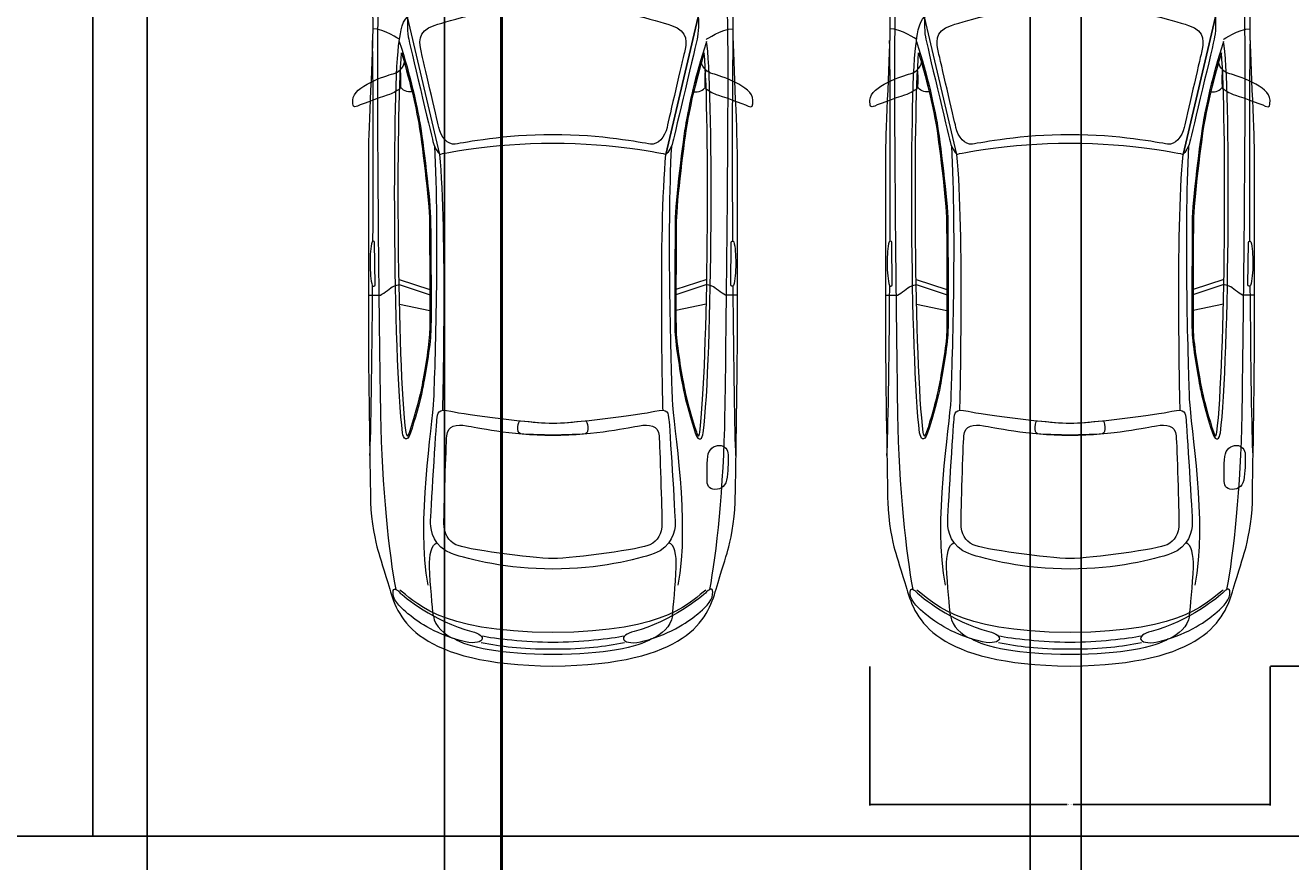
# Model space of a CAD drawing. Units: inches. Extents: x 1770 to 2988, y 1161 to 3221.
# Tile 3 of 44: x 2439 to 2663, y 1319 to 1467. Entities that reach past the tile are written whole.
import ezdxf

# ---------------------------------------------------------------- set-up
doc = ezdxf.new("R2010")
doc.units = ezdxf.units.IN
for name, color, linetype, lineweight in [('A-ANNO-DIMS', 2, 'Continuous', 18), ('AUDI', 8, 'Continuous', 13), ('C-PROP', 7, 'Continuous', 25), ('C-SITE-PAVE', 8, 'Continuous', 18)]:
    doc.layers.add(name, color=color, linetype=linetype, lineweight=lineweight)
doc.styles.get("Standard").update_dxf_attribs({"font": 'arial.ttf'})
doc.dimstyles.get("Standard").update_dxf_attribs({"dimtxt": 0.18, "dimasz": 0.18, "dimexe": 0.18, "dimexo": 0.0625, "dimgap": 0.09, "dimtad": 0, "dimtih": 1, "dimtoh": 1, "dimdec": 4, "dimzin": 0, "dimdsep": 46, "dimtxsty": 'Standard', "dimcen": 0.09, "dimadec": 0, "dimazin": 0, "dimtfac": 1, "dimtdec": 4, "dimtofl": 0, "dimtmove": 0, "dimatfit": 3, "dimfxl": 1, "dimtolj": 1, "dimtzin": 0, "dimarcsym": 0})

# ---------------------------------------------------------------- blocks, each defined once
blk = doc.blocks.new('CAR-SEDAN-PLAN')
for points, knots in [([(35.35, 0), (11.45, 0.26), (7.98, 8.3), (6.52, 13.59), (6.52, 13.59), (5.56, 16.72), (4.79, 19.21), (4.41, 20.48), (4.41, 20.48), (4.03, 21.76), (3.2, 25.65), (3.14, 28.9), (3.14, 28.9), (3.07, 32.16), (2.76, 51.56), (2.76, 56.91), (2.76, 56.91), (2.76, 62.27), (2.76, 87.35), (2.76, 90.92), (2.76, 90.92), (2.76, 94.49), (3.52, 108.72), (3.52, 113.25), (3.52, 113.25), (3.52, 117.78), (2.76, 123.46), (2.76, 125.81), (2.76, 125.81), (2.76, 128.17), (3.2, 140.62), (3.39, 143.36), (3.39, 143.36), (3.58, 146.1), (4.61, 147.66), (5.5, 149.61), (5.5, 149.61), (8.94, 157.2), (17.74, 161.35), (18.69, 161.99), (18.69, 161.99), (19.65, 162.63), (20.67, 162.97), (21.88, 162.97), (21.88, 162.97), (23.1, 162.97), (23.41, 162.37), (23.92, 162.5), (23.92, 162.5), (24.43, 162.63), (25.7, 162.97), (27.11, 162.97), (27.11, 162.97), (28.52, 162.97), (35.35, 162.97), (35.35, 162.97), (35.35, 162.97), (35.35, 162.97), (42.18, 162.97), (43.59, 162.97), (43.59, 162.97), (45, 162.97), (46.27, 162.63), (46.78, 162.5), (46.78, 162.5), (47.29, 162.37), (47.6, 162.97), (48.82, 162.97), (48.82, 162.97), (50.04, 162.97), (51.05, 162.63), (52.01, 161.99), (52.01, 161.99), (52.96, 161.35), (61.76, 157.2), (65.21, 149.61), (65.21, 149.61), (66.09, 147.66), (67.12, 146.1), (67.31, 143.36), (67.31, 143.36), (67.5, 140.62), (67.95, 128.17), (67.95, 125.81), (67.95, 125.81), (67.95, 123.46), (67.18, 117.78), (67.18, 113.25), (67.18, 113.25), (67.18, 108.72), (67.95, 94.49), (67.95, 90.92), (67.95, 90.92), (67.95, 87.35), (67.95, 62.27), (67.95, 56.91), (67.95, 56.91), (67.95, 51.56), (67.63, 32.16), (67.57, 28.9), (67.57, 28.9), (67.5, 25.65), (66.67, 21.76), (66.29, 20.48), (66.29, 20.48), (65.91, 19.21), (65.14, 16.72), (64.19, 13.59), (64.19, 13.59), (62.72, 8.3), (59.25, 0.26), (35.35, 0)], [0, 0, 0, 0, 0.035714, 0.035714, 0.035714, 0.035714, 0.071429, 0.071429, 0.071429, 0.071429, 0.107143, 0.107143, 0.107143, 0.107143, 0.142857, 0.142857, 0.142857, 0.142857, 0.178571, 0.178571, 0.178571, 0.178571, 0.214286, 0.214286, 0.214286, 0.214286, 0.25, 0.25, 0.25, 0.25, 0.285714, 0.285714, 0.285714, 0.285714, 0.321429, 0.321429, 0.321429, 0.321429, 0.357143, 0.357143, 0.357143, 0.357143, 0.392857, 0.392857, 0.392857, 0.392857, 0.428571, 0.428571, 0.428571, 0.428571, 0.464286, 0.464286, 0.464286, 0.464286, 0.5, 0.5, 0.5, 0.5, 0.535714, 0.535714, 0.535714, 0.535714, 0.571429, 0.571429, 0.571429, 0.571429, 0.607143, 0.607143, 0.607143, 0.607143, 0.642857, 0.642857, 0.642857, 0.642857, 0.678571, 0.678571, 0.678571, 0.678571, 0.714286, 0.714286, 0.714286, 0.714286, 0.75, 0.75, 0.75, 0.75, 0.785714, 0.785714, 0.785714, 0.785714, 0.821429, 0.821429, 0.821429, 0.821429, 0.857143, 0.857143, 0.857143, 0.857143, 0.892857, 0.892857, 0.892857, 0.892857, 0.928571, 0.928571, 0.928571, 0.928571, 0.964286, 0.964286, 0.964286, 0.964286, 1, 1, 1, 1]), ([(7.64, 13.52), (6.44, 19.53), (5.16, 31.7), (4.94, 44.37), (4.94, 44.37), (4.72, 57.04), (4.17, 105.75), (4.5, 116.02), (4.5, 116.02), (4.83, 126.28), (5.01, 139.24), (6.83, 148.05)], [0, 0, 0, 0, 0.333333, 0.333333, 0.333333, 0.333333, 0.666667, 0.666667, 0.666667, 0.666667, 1, 1, 1, 1]), ([(63.07, 13.52), (64.27, 19.53), (65.54, 31.7), (65.76, 44.37), (65.76, 44.37), (65.98, 57.04), (66.53, 105.75), (66.2, 116.02), (66.2, 116.02), (65.87, 126.28), (65.69, 139.24), (63.87, 148.05)], [0, 0, 0, 0, 0.333333, 0.333333, 0.333333, 0.333333, 0.666667, 0.666667, 0.666667, 0.666667, 1, 1, 1, 1]), ([(35.35, 92.33), (46.17, 92.33), (55.33, 90.37), (55.33, 90.37), (55.33, 90.37), (55.33, 90.37), (61.04, 114.67), (61.04, 114.67), (61.04, 114.67), (58.76, 116.14), (55.78, 121.11), (35.35, 121.11), (35.35, 121.11), (14.92, 121.11), (11.94, 116.14), (9.66, 114.67), (9.66, 114.67), (9.66, 114.67), (15.37, 90.37), (15.37, 90.37), (15.37, 90.37), (15.37, 90.37), (24.53, 92.33), (35.35, 92.33)], [0, 0, 0, 0, 0.166667, 0.166667, 0.166667, 0.166667, 0.333333, 0.333333, 0.333333, 0.333333, 0.5, 0.5, 0.5, 0.5, 0.666667, 0.666667, 0.666667, 0.666667, 0.833333, 0.833333, 0.833333, 0.833333, 1, 1, 1, 1]), ([(35.35, 92.33), (46.17, 92.33), (55.33, 90.37), (55.33, 90.37), (55.33, 90.37), (55.33, 90.37), (61.04, 114.67), (61.04, 114.67), (61.04, 114.67), (58.76, 116.14), (55.78, 121.11), (35.35, 121.11), (35.35, 121.11), (14.92, 121.11), (11.94, 116.14), (9.66, 114.67), (9.66, 114.67), (9.66, 114.67), (15.37, 90.37), (15.37, 90.37), (15.37, 90.37), (15.37, 90.37), (24.53, 92.33), (35.35, 92.33)], [0, 0, 0, 0, 0.166667, 0.166667, 0.166667, 0.166667, 0.333333, 0.333333, 0.333333, 0.333333, 0.5, 0.5, 0.5, 0.5, 0.666667, 0.666667, 0.666667, 0.666667, 0.833333, 0.833333, 0.833333, 0.833333, 1, 1, 1, 1]), ([(9.66, 114.67), (9.66, 114.67), (15.37, 90.37), (15.37, 90.37), (15.37, 90.37), (15.37, 90.37), (14.48, 91.26), (14.15, 92.64), (14.15, 92.64), (13.82, 94.03), (10.04, 109.86), (9.79, 111.17), (9.79, 111.17), (9.55, 112.47), (9.66, 114.67), (9.66, 114.67)], [0, 0, 0, 0, 0.25, 0.25, 0.25, 0.25, 0.5, 0.5, 0.5, 0.5, 0.75, 0.75, 0.75, 0.75, 1, 1, 1, 1]), ([(9.66, 114.67), (9.66, 114.67), (15.37, 90.37), (15.37, 90.37), (15.37, 90.37), (15.37, 90.37), (14.48, 91.26), (14.15, 92.64), (14.15, 92.64), (13.82, 94.03), (10.04, 109.86), (9.79, 111.17), (9.79, 111.17), (9.55, 112.47), (9.66, 114.67), (9.66, 114.67)], [0, 0, 0, 0, 0.25, 0.25, 0.25, 0.25, 0.5, 0.5, 0.5, 0.5, 0.75, 0.75, 0.75, 0.75, 1, 1, 1, 1]), ([(35.35, 93.86), (43.94, 93.86), (50.97, 92.45), (52.59, 92.2), (52.59, 92.2), (53.92, 92), (55.15, 93.44), (55.52, 95.16), (55.52, 95.16), (55.89, 96.88), (58.26, 106.94), (58.59, 108.38), (58.59, 108.38), (58.92, 109.82), (59.47, 112.19), (56.31, 113.17), (56.31, 113.17), (53.15, 114.15), (47.56, 116.15), (35.35, 116.15), (35.35, 116.15), (23.15, 116.15), (17.55, 114.15), (14.39, 113.17), (14.39, 113.17), (11.23, 112.19), (11.79, 109.82), (12.11, 108.38), (12.11, 108.38), (12.44, 106.94), (14.81, 96.88), (15.18, 95.16), (15.18, 95.16), (15.55, 93.44), (16.78, 92), (18.11, 92.2), (18.11, 92.2), (19.74, 92.45), (26.76, 93.86), (35.35, 93.86)], [0, 0, 0, 0, 0.1, 0.1, 0.1, 0.1, 0.2, 0.2, 0.2, 0.2, 0.3, 0.3, 0.3, 0.3, 0.4, 0.4, 0.4, 0.4, 0.5, 0.5, 0.5, 0.5, 0.6, 0.6, 0.6, 0.6, 0.7, 0.7, 0.7, 0.7, 0.8, 0.8, 0.8, 0.8, 0.9, 0.9, 0.9, 0.9, 1, 1, 1, 1]), ([(61.04, 114.67), (61.04, 114.67), (55.33, 90.37), (55.33, 90.37), (55.33, 90.37), (55.33, 90.37), (56.23, 91.26), (56.55, 92.64), (56.55, 92.64), (56.88, 94.03), (60.66, 109.86), (60.91, 111.17), (60.91, 111.17), (61.15, 112.47), (61.04, 114.67), (61.04, 114.67)], [0, 0, 0, 0, 0.25, 0.25, 0.25, 0.25, 0.5, 0.5, 0.5, 0.5, 0.75, 0.75, 0.75, 0.75, 1, 1, 1, 1]), ([(8.78, 41.21), (8.91, 40.21), (9.53, 39.31), (10.19, 41.21), (10.19, 41.21), (10.85, 43.12), (11.93, 47.01), (12.26, 48.66), (12.26, 48.66), (12.59, 50.32), (13.58, 55.79), (13.75, 58.52), (13.75, 58.52), (13.92, 61.25), (13.75, 75.25), (13.75, 78.56), (13.75, 78.56), (13.75, 81.87), (12.34, 93.22), (11.85, 95.95), (11.85, 95.95), (11.35, 98.68), (10.27, 104.15), (8.2, 110.31), (8.2, 110.31), (6.96, 103.49), (7.13, 54.21), (8.78, 41.21)], [0, 0, 0, 0, 0.142857, 0.142857, 0.142857, 0.142857, 0.285714, 0.285714, 0.285714, 0.285714, 0.428571, 0.428571, 0.428571, 0.428571, 0.571429, 0.571429, 0.571429, 0.571429, 0.714286, 0.714286, 0.714286, 0.714286, 0.857143, 0.857143, 0.857143, 0.857143, 1, 1, 1, 1]), ([(61.92, 41.21), (61.79, 40.21), (61.17, 39.31), (60.51, 41.21), (60.51, 41.21), (59.85, 43.12), (58.77, 47.01), (58.44, 48.66), (58.44, 48.66), (58.11, 50.32), (57.12, 55.79), (56.95, 58.52), (56.95, 58.52), (56.79, 61.25), (56.95, 75.25), (56.95, 78.56), (56.95, 78.56), (56.95, 81.87), (58.36, 93.22), (58.86, 95.95), (58.86, 95.95), (59.35, 98.68), (60.43, 104.15), (62.5, 110.31), (62.5, 110.31), (63.74, 103.49), (63.57, 54.21), (61.92, 41.21)], [0, 0, 0, 0, 0.142857, 0.142857, 0.142857, 0.142857, 0.285714, 0.285714, 0.285714, 0.285714, 0.428571, 0.428571, 0.428571, 0.428571, 0.571429, 0.571429, 0.571429, 0.571429, 0.714286, 0.714286, 0.714286, 0.714286, 0.857143, 0.857143, 0.857143, 0.857143, 1, 1, 1, 1]), ([(9.41, 41.26), (9.41, 41.26), (9.41, 41.26), (9.41, 41.26), (9.41, 41.26), (9.46, 40.9), (9.56, 40.69), (9.63, 40.58), (9.63, 40.58), (9.71, 40.67), (9.84, 40.87), (10, 41.35), (10, 41.35), (10.65, 43.21), (11.72, 47.08), (12.06, 48.75), (12.06, 48.75), (12.46, 50.75), (13.39, 55.99), (13.54, 58.54), (13.54, 58.54), (13.66, 60.54), (13.6, 68.71), (13.56, 74.11), (13.56, 74.11), (13.56, 74.11), (13.54, 78.56), (13.54, 78.56), (13.54, 78.56), (13.54, 81.86), (12.12, 93.26), (11.64, 95.88), (11.64, 95.88), (10.85, 100.24), (9.82, 104.4), (8.6, 108.3), (8.6, 108.3), (7.63, 97), (7.88, 53.31), (9.41, 41.26)], [0, 0, 0, 0, 0.1, 0.1, 0.1, 0.1, 0.2, 0.2, 0.2, 0.2, 0.3, 0.3, 0.3, 0.3, 0.4, 0.4, 0.4, 0.4, 0.5, 0.5, 0.5, 0.5, 0.6, 0.6, 0.6, 0.6, 0.7, 0.7, 0.7, 0.7, 0.8, 0.8, 0.8, 0.8, 0.9, 0.9, 0.9, 0.9, 1, 1, 1, 1]), ([(61.29, 41.26), (61.29, 41.26), (61.29, 41.26), (61.29, 41.26), (61.29, 41.26), (61.24, 40.9), (61.14, 40.69), (61.07, 40.58), (61.07, 40.58), (60.99, 40.67), (60.86, 40.87), (60.7, 41.35), (60.7, 41.35), (60.05, 43.21), (58.98, 47.08), (58.64, 48.75), (58.64, 48.75), (58.24, 50.75), (57.32, 55.99), (57.16, 58.54), (57.16, 58.54), (57.04, 60.54), (57.1, 68.71), (57.14, 74.11), (57.14, 74.11), (57.14, 74.11), (57.16, 78.56), (57.16, 78.56), (57.16, 78.56), (57.16, 81.86), (58.59, 93.26), (59.06, 95.88), (59.06, 95.88), (59.85, 100.24), (60.88, 104.4), (62.1, 108.3), (62.1, 108.3), (63.07, 97), (62.82, 53.31), (61.29, 41.26)], [0, 0, 0, 0, 0.1, 0.1, 0.1, 0.1, 0.2, 0.2, 0.2, 0.2, 0.3, 0.3, 0.3, 0.3, 0.4, 0.4, 0.4, 0.4, 0.5, 0.5, 0.5, 0.5, 0.6, 0.6, 0.6, 0.6, 0.7, 0.7, 0.7, 0.7, 0.8, 0.8, 0.8, 0.8, 0.9, 0.9, 0.9, 0.9, 1, 1, 1, 1]), ([(8.34, 105.29), (8.03, 105), (7.63, 104.75), (7.11, 104.61), (7.11, 104.61), (5.83, 104.26), (0.07, 102.46), (0, 99.98), (0, 99.98), (0, 98.93), (0.02, 98.57), (0.85, 98.93), (0.85, 98.93), (1.67, 99.3), (5.81, 100.79), (6.5, 100.99), (6.5, 100.99), (7.13, 101.18), (8.06, 101.74), (8.4, 102.11), (8.4, 102.11), (8.48, 103.13), (8.47, 104.61), (8.34, 105.29)], [0, 0, 0, 0, 0.166667, 0.166667, 0.166667, 0.166667, 0.333333, 0.333333, 0.333333, 0.333333, 0.5, 0.5, 0.5, 0.5, 0.666667, 0.666667, 0.666667, 0.666667, 0.833333, 0.833333, 0.833333, 0.833333, 1, 1, 1, 1]), ([(8.34, 105.29), (8.47, 104.61), (8.48, 103.13), (8.4, 102.11), (8.4, 102.11), (8.43, 102.14), (8.47, 102.18), (8.49, 102.2), (8.49, 102.2), (8.67, 101.82), (9.61, 101.3), (10.48, 101.44), (10.48, 101.44), (10.36, 101.92), (9.1, 106.66), (9.1, 106.66), (9.1, 106.66), (9.05, 106.27), (8.8, 105.73), (8.34, 105.29)], [0, 0, 0, 0, 0.2, 0.2, 0.2, 0.2, 0.4, 0.4, 0.4, 0.4, 0.6, 0.6, 0.6, 0.6, 0.8, 0.8, 0.8, 0.8, 1, 1, 1, 1]), ([(62.36, 105.29), (62.23, 104.61), (62.22, 103.13), (62.3, 102.11), (62.3, 102.11), (62.27, 102.14), (62.24, 102.18), (62.22, 102.2), (62.22, 102.2), (62.03, 101.82), (61.09, 101.3), (60.22, 101.44), (60.22, 101.44), (60.34, 101.92), (61.6, 106.66), (61.6, 106.66), (61.6, 106.66), (61.66, 106.27), (61.9, 105.73), (62.36, 105.29)], [0, 0, 0, 0, 0.2, 0.2, 0.2, 0.2, 0.4, 0.4, 0.4, 0.4, 0.6, 0.6, 0.6, 0.6, 0.8, 0.8, 0.8, 0.8, 1, 1, 1, 1]), ([(62.36, 105.29), (62.67, 105), (63.07, 104.75), (63.59, 104.61), (63.59, 104.61), (64.87, 104.26), (70.63, 102.46), (70.7, 99.98), (70.7, 99.98), (70.7, 98.93), (70.68, 98.57), (69.86, 98.93), (69.86, 98.93), (69.03, 99.3), (64.89, 100.79), (64.21, 100.99), (64.21, 100.99), (63.57, 101.18), (62.64, 101.74), (62.3, 102.11), (62.3, 102.11), (62.22, 103.13), (62.23, 104.61), (62.36, 105.29)], [0, 0, 0, 0, 0.166667, 0.166667, 0.166667, 0.166667, 0.333333, 0.333333, 0.333333, 0.333333, 0.5, 0.5, 0.5, 0.5, 0.666667, 0.666667, 0.666667, 0.666667, 0.833333, 0.833333, 0.833333, 0.833333, 1, 1, 1, 1]), ([(14.41, 91.86), (15.27, 76.4), (14.46, 52.09), (14.27, 47.16), (14.27, 47.16), (14.09, 42.23), (11.07, 25.47), (13.28, 14.26)], [0, 0, 0, 0, 0.5, 0.5, 0.5, 0.5, 1, 1, 1, 1]), ([(56.29, 91.86), (55.44, 76.4), (56.24, 52.09), (56.43, 47.16), (56.43, 47.16), (56.61, 42.23), (59.63, 25.47), (57.42, 14.26)], [0, 0, 0, 0, 0.5, 0.5, 0.5, 0.5, 1, 1, 1, 1]), ([(3.92, 67.36), (3.92, 67.07), (3.53, 66.96), (3.44, 67.25), (3.44, 67.25), (3.17, 68.09), (3.04, 69.59), (3.04, 71.09), (3.04, 71.09), (3.04, 72.59), (3.13, 74.05), (3.39, 74.92), (3.39, 74.92), (3.48, 75.18), (3.84, 75.11), (3.84, 74.81), (3.84, 74.81), (3.84, 74.81), (3.92, 67.36), (3.92, 67.36)], [0, 0, 0, 0, 0.2, 0.2, 0.2, 0.2, 0.4, 0.4, 0.4, 0.4, 0.6, 0.6, 0.6, 0.6, 0.8, 0.8, 0.8, 0.8, 1, 1, 1, 1]), ([(66.78, 67.36), (66.78, 67.07), (67.18, 66.96), (67.27, 67.25), (67.27, 67.25), (67.53, 68.09), (67.66, 69.59), (67.66, 71.09), (67.66, 71.09), (67.66, 72.59), (67.58, 74.05), (67.31, 74.92), (67.31, 74.92), (67.22, 75.18), (66.87, 75.11), (66.87, 74.81), (66.87, 74.81), (66.87, 74.81), (66.78, 67.36), (66.78, 67.36)], [0, 0, 0, 0, 0.2, 0.2, 0.2, 0.2, 0.4, 0.4, 0.4, 0.4, 0.6, 0.6, 0.6, 0.6, 0.8, 0.8, 0.8, 0.8, 1, 1, 1, 1]), ([(2.76, 65.49), (2.76, 65.49), (4.19, 65.49), (4.66, 65.49), (4.66, 65.49), (5.14, 65.49), (6.39, 66.63), (6.96, 66.97), (6.96, 66.97), (7.54, 67.3), (8.17, 67.38), (8.17, 67.38)], [0, 0, 0, 0, 0.333333, 0.333333, 0.333333, 0.333333, 0.666667, 0.666667, 0.666667, 0.666667, 1, 1, 1, 1]), ([(67.95, 65.49), (67.95, 65.49), (66.51, 65.49), (66.04, 65.49), (66.04, 65.49), (65.57, 65.49), (64.32, 66.63), (63.74, 66.97), (63.74, 66.97), (63.16, 67.3), (62.53, 67.38), (62.53, 67.38)], [0, 0, 0, 0, 0.333333, 0.333333, 0.333333, 0.333333, 0.666667, 0.666667, 0.666667, 0.666667, 1, 1, 1, 1]), ([(35.35, 17.14), (43.39, 17.14), (50.14, 18.76), (53.24, 19.87), (53.24, 19.87), (56.34, 20.99), (56.96, 23.85), (56.96, 25.27), (56.96, 25.27), (56.96, 26.7), (55.97, 42.4), (55.85, 43.52), (55.85, 43.52), (55.72, 44.63), (55.78, 45.63), (53.36, 45.01), (53.36, 45.01), (50.95, 44.39), (38.36, 42.9), (35.35, 42.9), (35.35, 42.9), (32.35, 42.9), (19.76, 44.39), (17.34, 45.01), (17.34, 45.01), (14.92, 45.63), (14.98, 44.63), (14.86, 43.52), (14.86, 43.52), (14.73, 42.4), (13.74, 26.7), (13.74, 25.27), (13.74, 25.27), (13.74, 23.85), (14.36, 20.99), (17.46, 19.87), (17.46, 19.87), (20.56, 18.76), (27.32, 17.14), (35.35, 17.14)], [0, 0, 0, 0, 0.1, 0.1, 0.1, 0.1, 0.2, 0.2, 0.2, 0.2, 0.3, 0.3, 0.3, 0.3, 0.4, 0.4, 0.4, 0.4, 0.5, 0.5, 0.5, 0.5, 0.6, 0.6, 0.6, 0.6, 0.7, 0.7, 0.7, 0.7, 0.8, 0.8, 0.8, 0.8, 0.9, 0.9, 0.9, 0.9, 1, 1, 1, 1]), ([(35.35, 17.14), (43.39, 17.14), (50.14, 18.76), (53.24, 19.87), (53.24, 19.87), (56.34, 20.99), (56.96, 23.85), (56.96, 25.27), (56.96, 25.27), (56.96, 26.7), (55.97, 42.4), (55.85, 43.52), (55.85, 43.52), (55.72, 44.63), (55.78, 45.63), (53.36, 45.01), (53.36, 45.01), (50.95, 44.39), (38.36, 42.9), (35.35, 42.9), (35.35, 42.9), (32.35, 42.9), (19.76, 44.39), (17.34, 45.01), (17.34, 45.01), (14.92, 45.63), (14.98, 44.63), (14.86, 43.52), (14.86, 43.52), (14.73, 42.4), (13.74, 26.7), (13.74, 25.27), (13.74, 25.27), (13.74, 23.85), (14.36, 20.99), (17.46, 19.87), (17.46, 19.87), (20.56, 18.76), (27.32, 17.14), (35.35, 17.14)], [0, 0, 0, 0, 0.1, 0.1, 0.1, 0.1, 0.2, 0.2, 0.2, 0.2, 0.3, 0.3, 0.3, 0.3, 0.4, 0.4, 0.4, 0.4, 0.5, 0.5, 0.5, 0.5, 0.6, 0.6, 0.6, 0.6, 0.7, 0.7, 0.7, 0.7, 0.8, 0.8, 0.8, 0.8, 0.9, 0.9, 0.9, 0.9, 1, 1, 1, 1]), ([(35.35, 19), (39.16, 19), (51.13, 20.68), (52.5, 21.43), (52.5, 21.43), (53.86, 22.17), (54.61, 23.22), (54.61, 25.27), (54.61, 25.27), (54.61, 27.32), (54.23, 38.8), (54.11, 40.66), (54.11, 40.66), (53.99, 42.52), (52.31, 42.71), (50.64, 42.46), (50.64, 42.46), (48.96, 42.21), (43.07, 40.79), (35.35, 40.79), (35.35, 40.79), (27.63, 40.79), (21.74, 42.21), (20.07, 42.46), (20.07, 42.46), (18.39, 42.71), (16.72, 42.52), (16.59, 40.66), (16.59, 40.66), (16.47, 38.8), (16.1, 27.32), (16.1, 25.27), (16.1, 25.27), (16.1, 23.22), (16.84, 22.17), (18.21, 21.43), (18.21, 21.43), (19.57, 20.68), (31.54, 19), (35.35, 19)], [0, 0, 0, 0, 0.1, 0.1, 0.1, 0.1, 0.2, 0.2, 0.2, 0.2, 0.3, 0.3, 0.3, 0.3, 0.4, 0.4, 0.4, 0.4, 0.5, 0.5, 0.5, 0.5, 0.6, 0.6, 0.6, 0.6, 0.7, 0.7, 0.7, 0.7, 0.8, 0.8, 0.8, 0.8, 0.9, 0.9, 0.9, 0.9, 1, 1, 1, 1]), ([(35.35, 40.79), (35.35, 40.79), (39.9, 40.87), (41.09, 41.04), (41.09, 41.04), (41.83, 41.15), (41.48, 43.37), (41.13, 43.34), (41.13, 43.34), (38.95, 43.13), (37.12, 42.9), (35.35, 42.9), (35.35, 42.9), (33.58, 42.9), (31.75, 43.13), (29.57, 43.34), (29.57, 43.34), (29.22, 43.37), (28.87, 41.15), (29.61, 41.04), (29.61, 41.04), (30.8, 40.87), (35.35, 40.79), (35.35, 40.79)], [0, 0, 0, 0, 0.166667, 0.166667, 0.166667, 0.166667, 0.333333, 0.333333, 0.333333, 0.333333, 0.5, 0.5, 0.5, 0.5, 0.666667, 0.666667, 0.666667, 0.666667, 0.833333, 0.833333, 0.833333, 0.833333, 1, 1, 1, 1]), ([(62.61, 32.88), (62.53, 32.07), (62.82, 31.23), (63.99, 31.2), (63.99, 31.2), (65.17, 31.18), (65.98, 31.81), (66.15, 33.36), (66.15, 33.36), (66.32, 34.92), (66.32, 36.47), (66.32, 37.33), (66.32, 37.33), (66.32, 38.2), (65.72, 38.97), (64.77, 38.97), (64.77, 38.97), (63.82, 38.97), (62.87, 38.37), (62.7, 36.99), (62.7, 36.99), (62.53, 35.61), (62.61, 32.88), (62.61, 32.88)], [0, 0, 0, 0, 0.166667, 0.166667, 0.166667, 0.166667, 0.333333, 0.333333, 0.333333, 0.333333, 0.5, 0.5, 0.5, 0.5, 0.666667, 0.666667, 0.666667, 0.666667, 0.833333, 0.833333, 0.833333, 0.833333, 1, 1, 1, 1]), ([(14.24, 8.87), (14.05, 10.4), (13.69, 14.31), (13.55, 17.48), (13.55, 17.48), (13.46, 19.63), (13.92, 21.53), (14.85, 21.79)], [0, 0, 0, 0, 0.5, 0.5, 0.5, 0.5, 1, 1, 1, 1]), ([(56.46, 8.87), (56.65, 10.4), (57.01, 14.31), (57.15, 17.48), (57.15, 17.48), (57.24, 19.63), (56.78, 21.53), (55.85, 21.79)], [0, 0, 0, 0, 0.5, 0.5, 0.5, 0.5, 1, 1, 1, 1]), ([(21, 6.11), (14.38, 7.82), (9.01, 12.29), (8.18, 13.09), (8.18, 13.09), (7.46, 13.8), (7.01, 13.87), (7.12, 12.63), (7.12, 12.63), (7.23, 11.4), (8.78, 10.02), (9.74, 9.23), (9.74, 9.23), (10.95, 8.22), (14.29, 5.7), (19.21, 4.45), (19.21, 4.45), (21.09, 3.91), (22.44, 4.09), (22.8, 4.63), (22.8, 4.63), (23.15, 5.17), (22.32, 5.76), (21, 6.11)], [0, 0, 0, 0, 0.166667, 0.166667, 0.166667, 0.166667, 0.333333, 0.333333, 0.333333, 0.333333, 0.5, 0.5, 0.5, 0.5, 0.666667, 0.666667, 0.666667, 0.666667, 0.833333, 0.833333, 0.833333, 0.833333, 1, 1, 1, 1]), ([(62.4, 13.43), (60.03, 11.81), (55.98, 5.94), (35.35, 5.94), (35.35, 5.94), (14.73, 5.94), (10.67, 11.81), (8.3, 13.43)], [0, 0, 0, 0, 0.5, 0.5, 0.5, 0.5, 1, 1, 1, 1]), ([(49.7, 6.11), (56.32, 7.82), (61.69, 12.29), (62.52, 13.09), (62.52, 13.09), (63.25, 13.8), (63.69, 13.87), (63.58, 12.63), (63.58, 12.63), (63.47, 11.4), (61.92, 10.02), (60.97, 9.23), (60.97, 9.23), (59.75, 8.22), (56.42, 5.7), (51.49, 4.45), (51.49, 4.45), (49.61, 3.91), (48.26, 4.09), (47.91, 4.63), (47.91, 4.63), (47.55, 5.17), (48.38, 5.76), (49.7, 6.11)], [0, 0, 0, 0, 0.166667, 0.166667, 0.166667, 0.166667, 0.333333, 0.333333, 0.333333, 0.333333, 0.5, 0.5, 0.5, 0.5, 0.666667, 0.666667, 0.666667, 0.666667, 0.833333, 0.833333, 0.833333, 0.833333, 1, 1, 1, 1]), ([(52.75, 4.81), (50.45, 3.34), (44.44, 2.03), (35.35, 2.03), (35.35, 2.03), (26.26, 2.03), (20.25, 3.34), (17.95, 4.81)], [0, 0, 0, 0, 0.5, 0.5, 0.5, 0.5, 1, 1, 1, 1]), ([(48.01, 5.28), (45.61, 4.83), (40.16, 4.17), (35.35, 4.17), (35.35, 4.17), (30.54, 4.17), (25.09, 4.83), (22.7, 5.28)], [0, 0, 0, 0, 0.5, 0.5, 0.5, 0.5, 1, 1, 1, 1]), ([(48.01, 4.08), (44.31, 3.43), (41.37, 2.96), (35.35, 2.96), (35.35, 2.96), (29.33, 2.96), (26.39, 3.43), (22.7, 4.08)], [0, 0, 0, 0, 0.5, 0.5, 0.5, 0.5, 1, 1, 1, 1])]:
    blk.add_open_spline(points, degree=3, knots=knots)
for points in [[(8.16, 109.91), (8.28, 111.03), (8.55, 113.81), (9.66, 114.67)], [(8.25, 110.69), (8.25, 110.69), (5.57, 112.58), (3.51, 112.58)], [(62.45, 110.69), (62.45, 110.69), (65.13, 112.58), (67.19, 112.58)], [(3.55, 75.07), (3.63, 89.88), (3.62, 104.6), (3.47, 110.53)], [(67.15, 75.07), (67.07, 89.88), (67.08, 104.6), (67.23, 110.53)], [(15.89, 45.19), (15.89, 45.19), (16.68, 76.85), (15.37, 90.37)], [(54.81, 45.19), (54.81, 45.19), (54.02, 76.85), (55.33, 90.37)], [(3, 37.21), (3.21, 40.99), (3.39, 53.41), (3.5, 67.15)], [(8.16, 68.28), (8.16, 68.28), (13.61, 66.49), (13.61, 66.49)], [(8.17, 67.38), (8.17, 67.38), (13.82, 65.49), (13.82, 65.49)], [(62.53, 67.38), (62.53, 67.38), (56.88, 65.49), (56.88, 65.49)], [(62.54, 68.28), (62.54, 68.28), (57.09, 66.49), (57.09, 66.49)], [(67.7, 37.21), (67.49, 40.99), (67.31, 53.41), (67.21, 67.15)], [(8.24, 63.9), (8.24, 63.9), (13.61, 62.83), (13.61, 62.83)], [(62.46, 63.9), (62.46, 63.9), (57.09, 62.83), (57.09, 62.83)], [(14.24, 8.87), (14.45, 6.91), (16.37, 5.51), (17.62, 4.91)], [(56.46, 8.87), (56.26, 6.91), (54.33, 5.51), (53.08, 4.91)]]:
    blk.add_open_spline(points, degree=3)
blk = doc.blocks.new('*D50')
at = {"layer": 'A-ANNO-DIMS', "color": 0, "lineweight": -2, "transparency": 16777216}
for p, q in [((2659.16, 1516.52), (2683.72, 1516.52)), ((2683.54, 1516.34), (2683.54, 1435.22)), ((2683.54, 1353.73), (2683.54, 1434.85)), ((2659.16, 1353.55), (2683.72, 1353.55))]:
    blk.add_line(p, q, dxfattribs=at)
at = {"layer": 'A-ANNO-DIMS', "color": 0, "transparency": 16777216}
for points in [[(2683.51, 1516.34), (2683.57, 1516.34), (2683.54, 1516.52)], [(2683.51, 1353.73), (2683.57, 1353.73), (2683.54, 1353.55)]]:
    blk.add_solid(points, dxfattribs=at)
at = {"layer": 'Defpoints', "color": 0, "transparency": 16777216}
for p in [(2659.1, 1516.52), (2683.54, 1516.52), (2659.1, 1353.55)]:
    blk.add_point(p, dxfattribs=at)
at = {"layer": 'A-ANNO-DIMS', "color": 0, "transparency": 16777216, "insert": (2683.54, 1435.04), "char_height": 0.18, "attachment_point": 5}
blk.add_mtext('\\A1;SEDAN 163 TYP.', dxfattribs=at)
blk = doc.blocks.new('*D51')
at = {"layer": 'A-ANNO-DIMS', "color": 0, "lineweight": -2, "transparency": 16777216}
for p, q in [((2588.4, 1353.49), (2588.4, 1328.93)), ((2659.1, 1353.49), (2659.1, 1328.93)), ((2588.58, 1329.11), (2623.22, 1329.11)), ((2658.92, 1329.11), (2624.28, 1329.11))]:
    blk.add_line(p, q, dxfattribs=at)
at = {"layer": 'A-ANNO-DIMS', "color": 0, "transparency": 16777216}
for points in [[(2588.58, 1329.14), (2588.58, 1329.08), (2588.4, 1329.11)], [(2658.92, 1329.14), (2658.92, 1329.08), (2659.1, 1329.11)]]:
    blk.add_solid(points, dxfattribs=at)
at = {"layer": 'Defpoints', "color": 0, "transparency": 16777216}
for p in [(2588.4, 1353.55), (2659.1, 1353.55), (2659.1, 1329.11)]:
    blk.add_point(p, dxfattribs=at)
at = {"layer": 'A-ANNO-DIMS', "color": 0, "transparency": 16777216, "insert": (2623.75, 1329.11), "char_height": 0.18, "attachment_point": 5}
blk.add_mtext('\\A1;71 TYP.', dxfattribs=at)
blk = doc.blocks.new('*D60')
at = {"layer": 'A-ANNO-DIMS', "color": 0, "lineweight": -2, "transparency": 16777216}
for p, q in [((2151.7, 1610.14), (2151.7, 1165.57)), ((2625.7, 1610.14), (2625.7, 1165.57)), ((2151.88, 1165.75), (2388.4, 1165.75)), ((2625.52, 1165.75), (2388.99, 1165.75))]:
    blk.add_line(p, q, dxfattribs=at)
at = {"layer": 'A-ANNO-DIMS', "color": 0, "transparency": 16777216}
for points in [[(2151.88, 1165.78), (2151.88, 1165.72), (2151.7, 1165.75)], [(2625.52, 1165.78), (2625.52, 1165.72), (2625.7, 1165.75)]]:
    blk.add_solid(points, dxfattribs=at)
at = {"layer": 'Defpoints', "color": 0, "transparency": 16777216}
for p in [(2151.7, 1610.2), (2625.7, 1610.2), (2625.7, 1165.75)]:
    blk.add_point(p, dxfattribs=at)
at = {"layer": 'A-ANNO-DIMS', "color": 0, "transparency": 16777216, "insert": (2388.7, 1165.75), "char_height": 0.18, "attachment_point": 5}
blk.add_mtext('\\A1;474', dxfattribs=at)
blk = doc.blocks.new('*D63')
at = {"layer": 'A-ANNO-DIMS', "color": 0, "lineweight": -2, "transparency": 16777216}
for p, q in [((2352.17, 1323.59), (2352.17, 2570.7)), ((2352.35, 2570.52), (2401.24, 2570.52)), ((2450.91, 2570.52), (2402.02, 2570.52)), ((2451.09, 1323.59), (2451.09, 2570.7))]:
    blk.add_line(p, q, dxfattribs=at)
at = {"layer": 'A-ANNO-DIMS', "color": 0, "transparency": 16777216}
for points in [[(2352.35, 2570.55), (2352.35, 2570.49), (2352.17, 2570.52)], [(2450.91, 2570.55), (2450.91, 2570.49), (2451.09, 2570.52)]]:
    blk.add_solid(points, dxfattribs=at)
at = {"layer": 'Defpoints', "color": 0, "transparency": 16777216}
for p in [(2451.09, 2570.52), (2352.17, 1323.53), (2451.09, 1323.53)]:
    blk.add_point(p, dxfattribs=at)
at = {"layer": 'A-ANNO-DIMS', "color": 0, "transparency": 16777216, "insert": (2401.63, 2570.52), "char_height": 0.18, "attachment_point": 5}
blk.add_mtext('\\A1;98.93', dxfattribs=at)
blk = doc.blocks.new('*D74')
at = {"layer": 'A-ANNO-DIMS', "color": 0, "lineweight": -2, "transparency": 16777216}
for p, q in [((2523.42, 2097.48), (2523.42, 1165.57)), ((2616.7, 2097.48), (2616.7, 1165.57)), ((2523.6, 1165.75), (2569.66, 1165.75)), ((2616.52, 1165.75), (2570.45, 1165.75))]:
    blk.add_line(p, q, dxfattribs=at)
at = {"layer": 'A-ANNO-DIMS', "color": 0, "transparency": 16777216}
for points in [[(2523.6, 1165.78), (2523.6, 1165.72), (2523.42, 1165.75)], [(2616.52, 1165.78), (2616.52, 1165.72), (2616.7, 1165.75)]]:
    blk.add_solid(points, dxfattribs=at)
at = {"layer": 'Defpoints', "color": 0, "transparency": 16777216}
for p in [(2523.42, 2097.54), (2616.7, 2097.54), (2616.7, 1165.75)]:
    blk.add_point(p, dxfattribs=at)
at = {"layer": 'A-ANNO-DIMS', "color": 0, "transparency": 16777216, "insert": (2570.06, 1165.75), "char_height": 0.18, "attachment_point": 5}
blk.add_mtext('\\A1;93.28', dxfattribs=at)
blk = doc.blocks.new('*D77')
at = {"layer": 'A-ANNO-DIMS', "color": 0, "lineweight": -2, "transparency": 16777216}
for p, q in [((2460.7, 1710.64), (2460.7, 1165.57)), ((2616.7, 1710.64), (2616.7, 1165.57)), ((2460.88, 1165.75), (2538.42, 1165.75)), ((2616.52, 1165.75), (2538.98, 1165.75))]:
    blk.add_line(p, q, dxfattribs=at)
at = {"layer": 'A-ANNO-DIMS', "color": 0, "transparency": 16777216}
for points in [[(2460.88, 1165.78), (2460.88, 1165.72), (2460.7, 1165.75)], [(2616.52, 1165.78), (2616.52, 1165.72), (2616.7, 1165.75)]]:
    blk.add_solid(points, dxfattribs=at)
at = {"layer": 'Defpoints', "color": 0, "transparency": 16777216}
for p in [(2460.7, 1710.7), (2616.7, 1710.7), (2616.7, 1165.75)]:
    blk.add_point(p, dxfattribs=at)
at = {"layer": 'A-ANNO-DIMS', "color": 0, "transparency": 16777216, "insert": (2538.7, 1165.75), "char_height": 0.18, "attachment_point": 5}
blk.add_mtext('\\A1;156', dxfattribs=at)
blk = doc.blocks.new('*D85')
at = {"layer": 'A-ANNO-DIMS', "color": 0, "lineweight": -2, "transparency": 16777216}
for p, q in [((2513.2, 1773.14), (2513.2, 1165.57)), ((2523.2, 1773.14), (2523.2, 1165.57)), ((2513.38, 1165.75), (2517.99, 1165.75)), ((2523.02, 1165.75), (2518.41, 1165.75))]:
    blk.add_line(p, q, dxfattribs=at)
at = {"layer": 'A-ANNO-DIMS', "color": 0, "transparency": 16777216}
for points in [[(2513.38, 1165.78), (2513.38, 1165.72), (2513.2, 1165.75)], [(2523.02, 1165.78), (2523.02, 1165.72), (2523.2, 1165.75)]]:
    blk.add_solid(points, dxfattribs=at)
at = {"layer": 'Defpoints', "color": 0, "transparency": 16777216}
for p in [(2513.2, 1773.2), (2523.2, 1773.2), (2523.2, 1165.75)]:
    blk.add_point(p, dxfattribs=at)
at = {"layer": 'A-ANNO-DIMS', "color": 0, "transparency": 16777216, "insert": (2518.2, 1165.75), "char_height": 0.18, "attachment_point": 5}
blk.add_mtext('\\A1;10', dxfattribs=at)

msp = doc.modelspace()

# ---------------------------------------------------------------- linework, layer by layer
at = {"layer": 'C-PROP'}
msp.add_lwpolyline([(1971.5344, 2506.2747), (2802.4374, 2506.2747), (2802.4374, 1323.5288), (1971.5344, 1323.5288)], close=True, dxfattribs=at)
at = {"layer": 'C-SITE-PAVE'}
msp.add_line((2451.0947, 1531.3388), (2451.0947, 1323.5288), dxfattribs=at)

# ---------------------------------------------------------------- block references
at = {"layer": 'AUDI'}
for p in [(2497.02, 1353.551), (2588.397, 1353.551)]:
    msp.add_blockref('CAR-SEDAN-PLAN', p, dxfattribs=at)

# ---------------------------------------------------------------- dimensions: what is measured, and where the dimension line sits
at = {"layer": 'A-ANNO-DIMS'}
for base, p1, p2, override, picture, middle in [((2451.0947, 2570.5247), (2352.1672, 1323.5288), (2451.0947, 1323.5288), {"dimdec": 2, "dimlfac": 1, "dimrnd": 0, "dimzin": 0, "dimdsep": 46, "dimlunit": 2}, '*D63', (2401.631, 2570.5247)), ((2616.696, 1165.752), (2523.4179, 2097.5443), (2616.696, 2097.5443), {"dimdec": 2, "dimlfac": 1, "dimrnd": 0, "dimzin": 0, "dimdsep": 46, "dimlunit": 2}, '*D74', (2570.0569, 1165.752)), ((2523.196, 1165.752), (2513.196, 1773.2021), (2523.196, 1773.2021), {"dimdec": 0, "dimlfac": 1, "dimrnd": 0, "dimzin": 0, "dimdsep": 46, "dimlunit": 2}, '*D85', (2518.196, 1165.752)), ((2616.696, 1165.752), (2460.696, 1710.7021), (2616.696, 1710.7021), {"dimdec": 0, "dimlfac": 1, "dimrnd": 0, "dimzin": 0, "dimdsep": 46, "dimlunit": 2}, '*D77', (2538.696, 1165.752)), ((2625.696, 1165.752), (2151.696, 1610.2021), (2625.696, 1610.2021), {"dimdec": 0, "dimlfac": 1, "dimrnd": 0, "dimzin": 0, "dimdsep": 46, "dimlunit": 2}, '*D60', (2388.696, 1165.752))]:
    dim = msp.add_linear_dim(base=base, p1=p1, p2=p2, dimstyle='Standard', override=override, dxfattribs=at)
    dim.commit()
    dim.dimension.update_dxf_attribs({"geometry": picture, "text_midpoint": middle})
dim = msp.add_linear_dim(base=(2683.5444, 1516.5237), p1=(2659.0986, 1353.5515), p2=(2659.0986, 1516.5237), angle=90, text='SEDAN <> TYP.', dimstyle='Standard', override={"dimdec": 0, "dimlfac": 1, "dimrnd": 0, "dimzin": 0, "dimdsep": 46, "dimlunit": 2}, dxfattribs=at)
dim.commit()
dim.dimension.update_dxf_attribs({"geometry": '*D50', "text_midpoint": (2683.5444, 1435.0376)})
dim = msp.add_linear_dim(base=(2659.0986, 1329.1056), p1=(2588.3971, 1353.5515), p2=(2659.0986, 1353.5515), text='<> TYP.', dimstyle='Standard', override={"dimdec": 0, "dimlfac": 1, "dimrnd": 0, "dimzin": 0, "dimdsep": 46, "dimlunit": 2}, dxfattribs=at)
dim.commit()
dim.dimension.update_dxf_attribs({"geometry": '*D51', "text_midpoint": (2623.7478, 1329.1056)})

doc.saveas('drawing.dxf')
